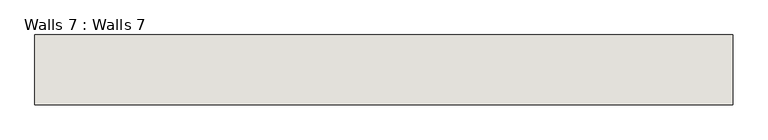
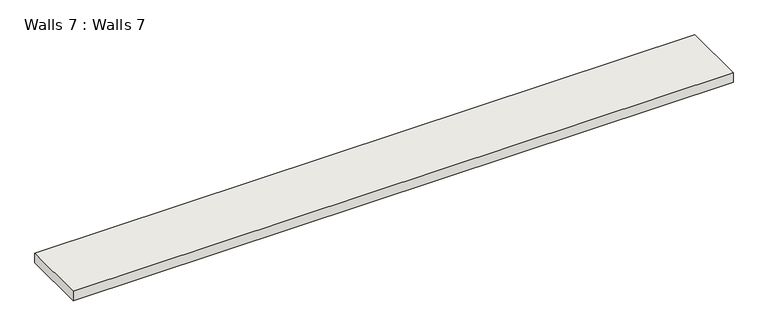
"""IFC4 building model written with IfcOpenShell, lengths in millimetres: wall geometry, Walls 7 : Walls 7."""

from ifc_helpers import new_model, si_unit, frame, origin, place, context, project, spatial, polyline, outline, extrude, source, transform, mapped, element, save


def walls_7_walls_7_ca1172f2(model_context):
    return source(origin(), model_context, "Body", "SweptSolid", [
        extrude(outline(polyline([(-14262.6019361, -6969.7875967), (-9260.4019361, -6969.7875967), (-9260.4019361, -7471.0562913), (-14262.6019361, -7471.0562913), (-14262.6019361, -6969.7875967)])), frame((0.0, 0.0, 1072.6182566), z_axis=(0.0, 0.0, 1.0), x_axis=(1.0, 0.0, 0.0)), (0.0, 0.0, 1.0), 75.3951578),
    ])


if __name__ == "__main__":
    model = new_model("IFC4")
    model_context = context("Model", 3, world=origin())
    ifc_project = project(units=[si_unit("LENGTHUNIT", "METRE", prefix="MILLI")], contexts=[model_context])
    site = spatial("IfcSite", under=ifc_project)
    building = spatial("IfcBuilding", under=site)
    placement = place(None, origin())
    walls_7_walls_7_shape = walls_7_walls_7_ca1172f2(model_context)
    element("IfcWall", 1, ObjectType="Walls 7 : Walls 7", at=placement, inside=building, context=model_context, shape_type="MappedRepresentation", body=[
        mapped(walls_7_walls_7_shape, transform((0.0, 0.0, 0.0), x_axis=(1.0, 0.0, 0.0), y_axis=(0.0, 1.0, 0.0), z_axis=(0.0, 0.0, 1.0))),
    ])
    save(model, "model.ifc")

# Revit data of these elements
# Element 1 (IfcWall, "Walls 7 : Walls 7")
#   Materials on its faces: "Default Wall"
# Materials
#   "Default Wall": colour RGB 80 80 80, transparency 0
